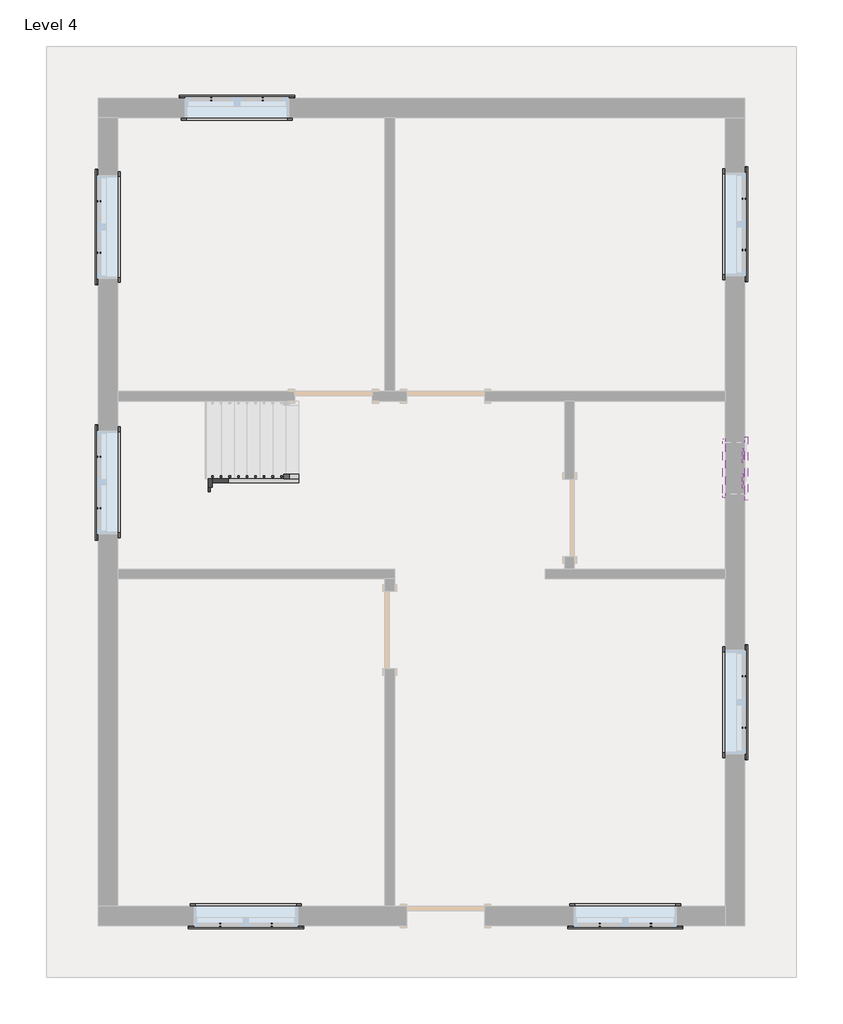
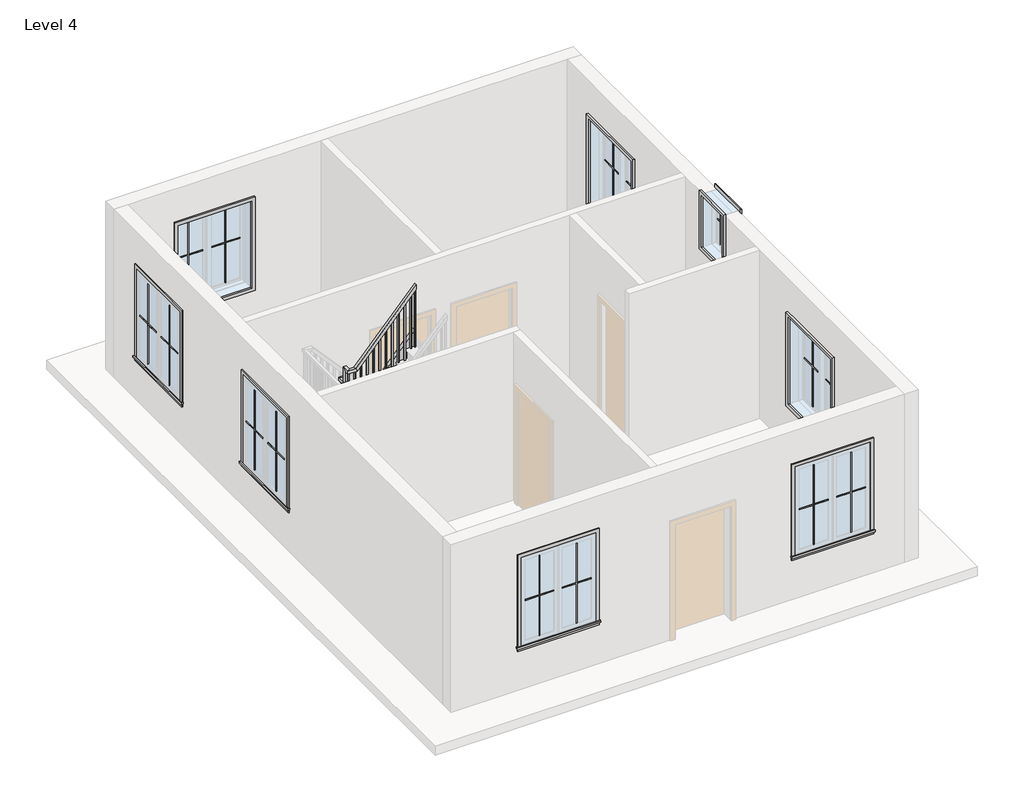
# One storey, part 2 of 2: 32 proxies, 3 members, 1 railing.
"""IFC4 building model written with IfcOpenShell, lengths in millimetres."""

from ifc_helpers import new_model, si_unit, frame, origin, place, context, project, spatial, polyline, outline, extrude, faceted_brep, transform, mapped, element, save
from components import muntin_pattern_2x2_muntin_pattern_2x2_6dad3731, muntin_pattern_2x2_muntin_pattern_2x2_a30a3345, muntin_pattern_2x2_muntin_pattern_2x2_53152e2c, muntin_pattern_2x2_muntin_pattern_2x2_e8f3e573, trim_window_exterior_flat_with_sill_92b9b949, trim_window_exterior_flat_with_sill_a665a915, trim_window_interior_flat_picture_frame_3bb882cf, trim_window_interior_flat_picture_frame_d485c387

model = new_model("IFC4")

# Units and contexts
model_context = context("Model", 3, world=origin())
ifc_project = project(units=[si_unit("LENGTHUNIT", "METRE", prefix="MILLI")], contexts=[model_context])

# Site, building, storey
site = spatial("IfcSite", under=ifc_project)
building = spatial("IfcBuilding", under=site)
storey = spatial("IfcBuildingStorey", under=building, Name="Level 4", Elevation=9144.0)

# Proxies
placement = place(None, origin())
muntin_pattern_2x2_muntin_pattern_2x2_shape = muntin_pattern_2x2_muntin_pattern_2x2_6dad3731(model_context)
element("IfcBuildingElementProxy", 1, Name="Muntin Pattern_2x2 : Muntin Pattern_2x2", ObjectType="Muntin Pattern_2x2 : Muntin Pattern_2x2", at=placement, inside=storey, context=model_context, shape_type="MappedRepresentation", body=[
    mapped(muntin_pattern_2x2_muntin_pattern_2x2_shape, transform((7785.1, 4733.925, 10128.25), x_axis=(-1.0, 0.0, 0.0), y_axis=(0.0, -1.0, 0.0), z_axis=(0.0, 0.0, 1.0))),
])
element("IfcBuildingElementProxy", 2, Name="Muntin Pattern_2x2 : Muntin Pattern_2x2", ObjectType="Muntin Pattern_2x2 : Muntin Pattern_2x2", at=placement, inside=storey, context=model_context, shape_type="MappedRepresentation", body=[
    mapped(muntin_pattern_2x2_muntin_pattern_2x2_shape, transform((3313.1125, 4733.925, 10128.25), x_axis=(-1.0, 0.0, 0.0), y_axis=(0.0, -1.0, 0.0), z_axis=(0.0, 0.0, 1.0))),
])
element("IfcBuildingElementProxy", 3, Name="Muntin Pattern_2x2 : Muntin Pattern_2x2", ObjectType="Muntin Pattern_2x2 : Muntin Pattern_2x2", at=placement, inside=storey, context=model_context, shape_type="MappedRepresentation", body=[
    mapped(muntin_pattern_2x2_muntin_pattern_2x2_shape, transform((8880.475, 13295.3125, 10128.25), x_axis=(0.0, -1.0, 0.0), y_axis=(1.0, 0.0, 0.0), z_axis=(0.0, 0.0, 1.0))),
])
element("IfcBuildingElementProxy", 4, Name="Muntin Pattern_2x2 : Muntin Pattern_2x2", ObjectType="Muntin Pattern_2x2 : Muntin Pattern_2x2", at=placement, inside=storey, context=model_context, shape_type="MappedRepresentation", body=[
    mapped(muntin_pattern_2x2_muntin_pattern_2x2_shape, transform((8880.475, 7662.8625, 10128.25), x_axis=(0.0, -1.0, 0.0), y_axis=(1.0, 0.0, 0.0), z_axis=(0.0, 0.0, 1.0))),
])
element("IfcBuildingElementProxy", 5, Name="Muntin Pattern_2x2 : Muntin Pattern_2x2", ObjectType="Muntin Pattern_2x2 : Muntin Pattern_2x2", at=placement, inside=storey, context=model_context, shape_type="MappedRepresentation", body=[
    mapped(muntin_pattern_2x2_muntin_pattern_2x2_shape, transform((1279.525, 12657.1375, 10128.25), x_axis=(0.0, 1.0, 0.0), y_axis=(-1.0, 0.0, 0.0), z_axis=(0.0, 0.0, 1.0))),
])
element("IfcBuildingElementProxy", 6, Name="Muntin Pattern_2x2 : Muntin Pattern_2x2", ObjectType="Muntin Pattern_2x2 : Muntin Pattern_2x2", at=placement, inside=storey, context=model_context, shape_type="MappedRepresentation", body=[
    mapped(muntin_pattern_2x2_muntin_pattern_2x2_shape, transform((1279.525, 9647.2375, 10128.25), x_axis=(0.0, 1.0, 0.0), y_axis=(-1.0, 0.0, 0.0), z_axis=(0.0, 0.0, 1.0))),
])
element("IfcBuildingElementProxy", 7, Name="Muntin Pattern_2x2 : Muntin Pattern_2x2", ObjectType="Muntin Pattern_2x2 : Muntin Pattern_2x2", at=placement, inside=storey, context=model_context, shape_type="MappedRepresentation", body=[
    mapped(muntin_pattern_2x2_muntin_pattern_2x2_shape, transform((2601.9125, 14468.475, 10128.25), x_axis=(1.0, 0.0, 0.0), y_axis=(0.0, 1.0, 0.0), z_axis=(0.0, 0.0, 1.0))),
])
muntin_pattern_2x2_muntin_pattern_2x2_2_shape = muntin_pattern_2x2_muntin_pattern_2x2_a30a3345(model_context)
element("IfcBuildingElementProxy", 8, Name="Muntin Pattern_2x2 : Muntin Pattern_2x2", ObjectType="Muntin Pattern_2x2 : Muntin Pattern_2x2", at=placement, inside=storey, context=model_context, shape_type="MappedRepresentation", body=[
    mapped(muntin_pattern_2x2_muntin_pattern_2x2_2_shape, transform((7178.675, 4733.925, 10128.25), x_axis=(1.0, 0.0, 0.0), y_axis=(0.0, 1.0, 0.0), z_axis=(0.0, 0.0, 1.0))),
])
element("IfcBuildingElementProxy", 9, Name="Muntin Pattern_2x2 : Muntin Pattern_2x2", ObjectType="Muntin Pattern_2x2 : Muntin Pattern_2x2", at=placement, inside=storey, context=model_context, shape_type="MappedRepresentation", body=[
    mapped(muntin_pattern_2x2_muntin_pattern_2x2_2_shape, transform((2706.6875, 4733.925, 10128.25), x_axis=(1.0, 0.0, 0.0), y_axis=(0.0, 1.0, 0.0), z_axis=(0.0, 0.0, 1.0))),
])
element("IfcBuildingElementProxy", 10, Name="Muntin Pattern_2x2 : Muntin Pattern_2x2", ObjectType="Muntin Pattern_2x2 : Muntin Pattern_2x2", at=placement, inside=storey, context=model_context, shape_type="MappedRepresentation", body=[
    mapped(muntin_pattern_2x2_muntin_pattern_2x2_2_shape, transform((8880.475, 12688.8875, 10128.25), x_axis=(0.0, 1.0, 0.0), y_axis=(-1.0, 0.0, 0.0), z_axis=(0.0, 0.0, 1.0))),
])
element("IfcBuildingElementProxy", 11, Name="Muntin Pattern_2x2 : Muntin Pattern_2x2", ObjectType="Muntin Pattern_2x2 : Muntin Pattern_2x2", at=placement, inside=storey, context=model_context, shape_type="MappedRepresentation", body=[
    mapped(muntin_pattern_2x2_muntin_pattern_2x2_2_shape, transform((8880.475, 7056.4375, 10128.25), x_axis=(0.0, 1.0, 0.0), y_axis=(-1.0, 0.0, 0.0), z_axis=(0.0, 0.0, 1.0))),
])
element("IfcBuildingElementProxy", 12, Name="Muntin Pattern_2x2 : Muntin Pattern_2x2", ObjectType="Muntin Pattern_2x2 : Muntin Pattern_2x2", at=placement, inside=storey, context=model_context, shape_type="MappedRepresentation", body=[
    mapped(muntin_pattern_2x2_muntin_pattern_2x2_2_shape, transform((1279.525, 13263.5625, 10128.25), x_axis=(0.0, -1.0, 0.0), y_axis=(1.0, 0.0, 0.0), z_axis=(0.0, 0.0, 1.0))),
])
element("IfcBuildingElementProxy", 13, Name="Muntin Pattern_2x2 : Muntin Pattern_2x2", ObjectType="Muntin Pattern_2x2 : Muntin Pattern_2x2", at=placement, inside=storey, context=model_context, shape_type="MappedRepresentation", body=[
    mapped(muntin_pattern_2x2_muntin_pattern_2x2_2_shape, transform((1279.525, 10253.6625, 10128.25), x_axis=(0.0, -1.0, 0.0), y_axis=(1.0, 0.0, 0.0), z_axis=(0.0, 0.0, 1.0))),
])
element("IfcBuildingElementProxy", 14, Name="Muntin Pattern_2x2 : Muntin Pattern_2x2", ObjectType="Muntin Pattern_2x2 : Muntin Pattern_2x2", at=placement, inside=storey, context=model_context, shape_type="MappedRepresentation", body=[
    mapped(muntin_pattern_2x2_muntin_pattern_2x2_2_shape, transform((3208.3375, 14468.475, 10128.25), x_axis=(-1.0, 0.0, 0.0), y_axis=(0.0, -1.0, 0.0), z_axis=(0.0, 0.0, 1.0))),
])
muntin_pattern_2x2_muntin_pattern_2x2_3_shape = muntin_pattern_2x2_muntin_pattern_2x2_53152e2c(model_context)
element("IfcBuildingElementProxy", 15, Name="Muntin Pattern_2x2 : Muntin Pattern_2x2", ObjectType="Muntin Pattern_2x2 : Muntin Pattern_2x2", at=placement, inside=storey, context=model_context, shape_type="MappedRepresentation", body=[
    mapped(muntin_pattern_2x2_muntin_pattern_2x2_3_shape, transform((8880.475, 10266.3625, 11347.45), x_axis=(0.0, -1.0, 0.0), y_axis=(1.0, 0.0, 0.0), z_axis=(0.0, 0.0, 1.0))),
])
muntin_pattern_2x2_muntin_pattern_2x2_4_shape = muntin_pattern_2x2_muntin_pattern_2x2_e8f3e573(model_context)
element("IfcBuildingElementProxy", 16, Name="Muntin Pattern_2x2 : Muntin Pattern_2x2", ObjectType="Muntin Pattern_2x2 : Muntin Pattern_2x2", at=placement, inside=storey, context=model_context, shape_type="MappedRepresentation", body=[
    mapped(muntin_pattern_2x2_muntin_pattern_2x2_4_shape, transform((8880.475, 9964.7375, 11347.45), x_axis=(0.0, 1.0, 0.0), y_axis=(-1.0, 0.0, 0.0), z_axis=(0.0, 0.0, 1.0))),
])
trim_window_exterior_flat_with_sill_shape = trim_window_exterior_flat_with_sill_92b9b949(model_context)
element("IfcBuildingElementProxy", 17, Name="Trim-Window-Exterior-Flat : with Sill", ObjectType="Trim-Window-Exterior-Flat : with Sill", at=placement, inside=storey, context=model_context, shape_type="MappedRepresentation", body=[
    mapped(trim_window_exterior_flat_with_sill_shape, transform((7481.8875, 4724.4, 11582.4), x_axis=(1.0, 0.0, 0.0), y_axis=(0.0, 0.0, 1.0), z_axis=(0.0, -1.0, 0.0))),
])
element("IfcBuildingElementProxy", 18, Name="Trim-Window-Exterior-Flat : with Sill", ObjectType="Trim-Window-Exterior-Flat : with Sill", at=placement, inside=storey, context=model_context, shape_type="MappedRepresentation", body=[
    mapped(trim_window_exterior_flat_with_sill_shape, transform((3009.9, 4724.4, 11582.4), x_axis=(1.0, 0.0, 0.0), y_axis=(0.0, 0.0, 1.0), z_axis=(0.0, -1.0, 0.0))),
])
element("IfcBuildingElementProxy", 19, Name="Trim-Window-Exterior-Flat : with Sill", ObjectType="Trim-Window-Exterior-Flat : with Sill", at=placement, inside=storey, context=model_context, shape_type="MappedRepresentation", body=[
    mapped(trim_window_exterior_flat_with_sill_shape, transform((8890.0, 12992.1, 11582.4), x_axis=(0.0, 1.0, 0.0), y_axis=(0.0, 0.0, 1.0), z_axis=(1.0, 0.0, 0.0))),
])
element("IfcBuildingElementProxy", 20, Name="Trim-Window-Exterior-Flat : with Sill", ObjectType="Trim-Window-Exterior-Flat : with Sill", at=placement, inside=storey, context=model_context, shape_type="MappedRepresentation", body=[
    mapped(trim_window_exterior_flat_with_sill_shape, transform((8890.0, 7359.65, 11582.4), x_axis=(0.0, 1.0, 0.0), y_axis=(0.0, 0.0, 1.0), z_axis=(1.0, 0.0, 0.0))),
])
element("IfcBuildingElementProxy", 21, Name="Trim-Window-Exterior-Flat : with Sill", ObjectType="Trim-Window-Exterior-Flat : with Sill", at=placement, inside=storey, context=model_context, shape_type="MappedRepresentation", body=[
    mapped(trim_window_exterior_flat_with_sill_shape, transform((1270.0, 12960.35, 11582.4), x_axis=(0.0, -1.0, 0.0), y_axis=(0.0, 0.0, 1.0), z_axis=(-1.0, 0.0, 0.0))),
])
element("IfcBuildingElementProxy", 22, Name="Trim-Window-Exterior-Flat : with Sill", ObjectType="Trim-Window-Exterior-Flat : with Sill", at=placement, inside=storey, context=model_context, shape_type="MappedRepresentation", body=[
    mapped(trim_window_exterior_flat_with_sill_shape, transform((1270.0, 9950.45, 11582.4), x_axis=(0.0, -1.0, 0.0), y_axis=(0.0, 0.0, 1.0), z_axis=(-1.0, 0.0, 0.0))),
])
element("IfcBuildingElementProxy", 23, Name="Trim-Window-Exterior-Flat : with Sill", ObjectType="Trim-Window-Exterior-Flat : with Sill", at=placement, inside=storey, context=model_context, shape_type="MappedRepresentation", body=[
    mapped(trim_window_exterior_flat_with_sill_shape, transform((2905.125, 14478.0, 11582.4), x_axis=(-1.0, 0.0, 0.0), y_axis=(0.0, 0.0, 1.0), z_axis=(0.0, 1.0, 0.0))),
])
trim_window_exterior_flat_with_sill_2_shape = trim_window_exterior_flat_with_sill_a665a915(model_context)
element("IfcBuildingElementProxy", 24, Name="Trim-Window-Exterior-Flat : with Sill", ObjectType="Trim-Window-Exterior-Flat : with Sill", at=placement, inside=storey, context=model_context, shape_type="MappedRepresentation", body=[
    mapped(trim_window_exterior_flat_with_sill_2_shape, transform((8890.0, 10115.55, 12192.0), x_axis=(0.0, 1.0, 0.0), y_axis=(0.0, 0.0, 1.0), z_axis=(1.0, 0.0, 0.0))),
])
trim_window_interior_flat_picture_frame_shape = trim_window_interior_flat_picture_frame_3bb882cf(model_context)
element("IfcBuildingElementProxy", 25, Name="Trim-Window-Interior-Flat : Picture Frame", ObjectType="Trim-Window-Interior-Flat : Picture Frame", at=placement, inside=storey, context=model_context, shape_type="MappedRepresentation", body=[
    mapped(trim_window_interior_flat_picture_frame_shape, transform((7481.8875, 4953.0, 11582.4), x_axis=(-1.0, 0.0, 0.0), y_axis=(0.0, 0.0, 1.0), z_axis=(0.0, 1.0, 0.0))),
])
element("IfcBuildingElementProxy", 26, Name="Trim-Window-Interior-Flat : Picture Frame", ObjectType="Trim-Window-Interior-Flat : Picture Frame", at=placement, inside=storey, context=model_context, shape_type="MappedRepresentation", body=[
    mapped(trim_window_interior_flat_picture_frame_shape, transform((3009.9, 4953.0, 11582.4), x_axis=(-1.0, 0.0, 0.0), y_axis=(0.0, 0.0, 1.0), z_axis=(0.0, 1.0, 0.0))),
])
element("IfcBuildingElementProxy", 27, Name="Trim-Window-Interior-Flat : Picture Frame", ObjectType="Trim-Window-Interior-Flat : Picture Frame", at=placement, inside=storey, context=model_context, shape_type="MappedRepresentation", body=[
    mapped(trim_window_interior_flat_picture_frame_shape, transform((8661.4, 12992.1, 11582.4), x_axis=(0.0, -1.0, 0.0), y_axis=(0.0, 0.0, 1.0), z_axis=(-1.0, 0.0, 0.0))),
])
element("IfcBuildingElementProxy", 28, Name="Trim-Window-Interior-Flat : Picture Frame", ObjectType="Trim-Window-Interior-Flat : Picture Frame", at=placement, inside=storey, context=model_context, shape_type="MappedRepresentation", body=[
    mapped(trim_window_interior_flat_picture_frame_shape, transform((8661.4, 7359.65, 11582.4), x_axis=(0.0, -1.0, 0.0), y_axis=(0.0, 0.0, 1.0), z_axis=(-1.0, 0.0, 0.0))),
])
element("IfcBuildingElementProxy", 29, Name="Trim-Window-Interior-Flat : Picture Frame", ObjectType="Trim-Window-Interior-Flat : Picture Frame", at=placement, inside=storey, context=model_context, shape_type="MappedRepresentation", body=[
    mapped(trim_window_interior_flat_picture_frame_shape, transform((1498.6, 12960.35, 11582.4), x_axis=(0.0, 1.0, 0.0), y_axis=(0.0, 0.0, 1.0), z_axis=(1.0, 0.0, 0.0))),
])
element("IfcBuildingElementProxy", 30, Name="Trim-Window-Interior-Flat : Picture Frame", ObjectType="Trim-Window-Interior-Flat : Picture Frame", at=placement, inside=storey, context=model_context, shape_type="MappedRepresentation", body=[
    mapped(trim_window_interior_flat_picture_frame_shape, transform((1498.6, 9950.45, 11582.4), x_axis=(0.0, 1.0, 0.0), y_axis=(0.0, 0.0, 1.0), z_axis=(1.0, 0.0, 0.0))),
])
element("IfcBuildingElementProxy", 31, Name="Trim-Window-Interior-Flat : Picture Frame", ObjectType="Trim-Window-Interior-Flat : Picture Frame", at=placement, inside=storey, context=model_context, shape_type="MappedRepresentation", body=[
    mapped(trim_window_interior_flat_picture_frame_shape, transform((2905.125, 14249.4, 11582.4), x_axis=(1.0, 0.0, 0.0), y_axis=(0.0, 0.0, 1.0), z_axis=(0.0, -1.0, 0.0))),
])
trim_window_interior_flat_picture_frame_2_shape = trim_window_interior_flat_picture_frame_d485c387(model_context)
element("IfcBuildingElementProxy", 32, Name="Trim-Window-Interior-Flat : Picture Frame", ObjectType="Trim-Window-Interior-Flat : Picture Frame", at=placement, inside=storey, context=model_context, shape_type="MappedRepresentation", body=[
    mapped(trim_window_interior_flat_picture_frame_2_shape, transform((8661.4, 10115.55, 12192.0), x_axis=(0.0, -1.0, 0.0), y_axis=(0.0, 0.0, 1.0), z_axis=(-1.0, 0.0, 0.0))),
])

# Members
element("IfcMember", 33, ObjectType="Stringer - 2\" Width", at=placement, inside=storey, context=model_context, shape_type="SweptSolid", body=[
    extrude(outline(polyline([(9144.0, 3632.2), (9418.6288314, 3632.2), (10547.5177203, 2616.2), (10091.8883192, 2616.2), (9144.0, 3469.2994873), (9144.0, 3632.2)])), frame((0.0, 9944.1, 0.0), z_axis=(0.0, 1.0, 0.0), x_axis=(0.0, 0.0, 1.0)), (0.0, 0.0, 1.0), 50.8),
])
element("IfcMember", 34, ObjectType="Stringer - 2\" Width", at=placement, inside=storey, context=model_context, shape_type="SweptSolid", body=[
    extrude(outline(polyline([(2565.4, 9994.9), (2616.2, 9994.9), (2616.2, 9893.3), (2565.4, 9893.3), (2565.4, 9994.9)])), frame((0.0, 0.0, 10270.0666667), z_axis=(0.0, 0.0, 1.0), x_axis=(1.0, 0.0, 0.0)), (0.0, 0.0, 1.0), 304.8),
])
element("IfcMember", 35, ObjectType="Stringer - 2\" Width", at=placement, inside=storey, context=model_context, shape_type="SweptSolid", body=[
    extrude(outline(polyline([(10773.2954981, 2565.4), (10317.666097, 2565.4), (11502.9994303, 3632.2), (11958.6288314, 3632.2), (10773.2954981, 2565.4)])), frame((0.0, 9842.5, 0.0), z_axis=(0.0, 1.0, 0.0), x_axis=(0.0, 0.0, 1.0)), (0.0, 0.0, 1.0), 50.8),
])

# Railing
element("IfcRailing", 36, ObjectType="Handrail - Rectangular", at=placement, inside=storey, context=model_context, shape_type="SolidModel", body=[
    faceted_brep([(3632.2, 9994.9, 10227.7333333), (3632.2, 9994.9, 10151.7950998), (3632.2, 10045.7, 10151.7950998), (3632.2, 10045.7, 10227.7333333), (2641.6, 9994.9, 11328.4), (2590.8, 9994.9, 11308.9062109), (2590.8, 10045.7, 11308.9062109), (2641.6, 10045.7, 11328.4), (2641.6, 9994.9, 11413.0666667), (2590.8, 9994.9, 11362.2666667), (2590.8, 10045.7, 11362.2666667), (2641.6, 10045.7, 11413.0666667), (2565.4, 9994.9, 11413.0666667), (2565.4, 9994.9, 11362.2666667), (2514.6, 10045.7, 11362.2666667), (2514.6, 10045.7, 11413.0666667), (2565.4, 9918.7, 11413.0666667), (2565.4, 9867.9, 11362.2666667), (2514.6, 9867.9, 11362.2666667), (2514.6, 9918.7, 11413.0666667), (2565.4, 9918.7, 11667.0666667), (2565.4, 9867.9, 11616.2666667), (2514.6, 9867.9, 11616.2666667), (2514.6, 9918.7, 11667.0666667), (2565.4, 9842.5, 11667.0666667), (2565.4, 9842.5, 11616.2666667), (2514.6, 9791.7, 11616.2666667), (2514.6, 9791.7, 11667.0666667), (2641.6, 9842.5, 11667.0666667), (2664.2244102, 9842.5, 11616.2666667), (2664.2244102, 9791.7, 11616.2666667), (2641.6, 9791.7, 11667.0666667), (3632.2, 9842.5, 12767.7333333), (3632.2, 9791.7, 12767.7333333), (3632.2, 9791.7, 12691.7950998), (3632.2, 9842.5, 12691.7950998)], [[[0, 1, 2, 3]], [[1, 0, 4, 5]], [[2, 1, 5, 6]], [[3, 2, 6, 7]], [[0, 3, 7, 4]], [[5, 4, 8, 9]], [[6, 5, 9, 10]], [[7, 6, 10, 11]], [[4, 7, 11, 8]], [[9, 8, 12, 13]], [[10, 9, 13, 14]], [[11, 10, 14, 15]], [[8, 11, 15, 12]], [[13, 12, 16, 17]], [[14, 13, 17, 18]], [[15, 14, 18, 19]], [[12, 15, 19, 16]], [[17, 16, 20, 21]], [[18, 17, 21, 22]], [[19, 18, 22, 23]], [[16, 19, 23, 20]], [[21, 20, 24, 25]], [[22, 21, 25, 26]], [[23, 22, 26, 27]], [[20, 23, 27, 24]], [[25, 24, 28, 29]], [[26, 25, 29, 30]], [[27, 26, 30, 31]], [[24, 27, 31, 28]], [[32, 33, 34, 35]], [[29, 28, 32, 35]], [[30, 29, 35, 34]], [[31, 30, 34, 33]], [[28, 31, 33, 32]]]),
    extrude(outline(polyline([(12596.5450998, 3546.475), (11684.0, 3546.475), (11684.0, 3565.525), (12617.7117665, 3565.525), (12596.5450998, 3546.475)])), frame((0.0, 9807.575, 0.0), z_axis=(0.0, 1.0, 0.0), x_axis=(0.0, 0.0, 1.0)), (0.0, 0.0, 1.0), 19.05),
    extrude(outline(polyline([(12483.6562109, 3444.875), (11514.6666667, 3444.875), (11514.6666667, 3463.925), (12504.8228776, 3463.925), (12483.6562109, 3444.875)])), frame((0.0, 9807.575, 0.0), z_axis=(0.0, 1.0, 0.0), x_axis=(0.0, 0.0, 1.0)), (0.0, 0.0, 1.0), 19.05),
    extrude(outline(polyline([(12370.767322, 3343.275), (11514.6666667, 3343.275), (11514.6666667, 3362.325), (12391.9339887, 3362.325), (12370.767322, 3343.275)])), frame((0.0, 9807.575, 0.0), z_axis=(0.0, 1.0, 0.0), x_axis=(0.0, 0.0, 1.0)), (0.0, 0.0, 1.0), 19.05),
    extrude(outline(polyline([(12257.8784332, 3241.675), (11345.3333333, 3241.675), (11345.3333333, 3260.725), (12279.0450998, 3260.725), (12257.8784332, 3241.675)])), frame((0.0, 9807.575, 0.0), z_axis=(0.0, 1.0, 0.0), x_axis=(0.0, 0.0, 1.0)), (0.0, 0.0, 1.0), 19.05),
    extrude(outline(polyline([(12144.9895443, 3140.075), (11176.0, 3140.075), (11176.0, 3159.125), (12166.1562109, 3159.125), (12144.9895443, 3140.075)])), frame((0.0, 9807.575, 0.0), z_axis=(0.0, 1.0, 0.0), x_axis=(0.0, 0.0, 1.0)), (0.0, 0.0, 1.0), 19.05),
    extrude(outline(polyline([(12032.1006554, 3038.475), (11176.0, 3038.475), (11176.0, 3057.525), (12053.267322, 3057.525), (12032.1006554, 3038.475)])), frame((0.0, 9807.575, 0.0), z_axis=(0.0, 1.0, 0.0), x_axis=(0.0, 0.0, 1.0)), (0.0, 0.0, 1.0), 19.05),
    extrude(outline(polyline([(11919.2117665, 2936.875), (11006.6666667, 2936.875), (11006.6666667, 2955.925), (11940.3784332, 2955.925), (11919.2117665, 2936.875)])), frame((0.0, 9807.575, 0.0), z_axis=(0.0, 1.0, 0.0), x_axis=(0.0, 0.0, 1.0)), (0.0, 0.0, 1.0), 19.05),
    extrude(outline(polyline([(11806.3228776, 2835.275), (10837.3333333, 2835.275), (10837.3333333, 2854.325), (11827.4895443, 2854.325), (11806.3228776, 2835.275)])), frame((0.0, 9807.575, 0.0), z_axis=(0.0, 1.0, 0.0), x_axis=(0.0, 0.0, 1.0)), (0.0, 0.0, 1.0), 19.05),
    extrude(outline(polyline([(11693.4339887, 2733.675), (10837.3333333, 2733.675), (10837.3333333, 2752.725), (11714.6006554, 2752.725), (11693.4339887, 2733.675)])), frame((0.0, 9807.575, 0.0), z_axis=(0.0, 1.0, 0.0), x_axis=(0.0, 0.0, 1.0)), (0.0, 0.0, 1.0), 19.05),
    extrude(outline(polyline([(11580.5450998, 2632.075), (10668.0, 2632.075), (10668.0, 2651.125), (11601.7117665, 2651.125), (11580.5450998, 2632.075)])), frame((0.0, 9807.575, 0.0), z_axis=(0.0, 1.0, 0.0), x_axis=(0.0, 0.0, 1.0)), (0.0, 0.0, 1.0), 19.05),
    extrude(outline(polyline([(2549.525, 9928.225), (2549.525, 9909.175), (2530.475, 9909.175), (2530.475, 9928.225), (2549.525, 9928.225)])), frame((0.0, 0.0, 10498.6666667), z_axis=(0.0, 0.0, 1.0), x_axis=(1.0, 0.0, 0.0)), (0.0, 0.0, 1.0), 863.6),
    extrude(outline(polyline([(2625.725, 10010.775), (2606.675, 10010.775), (2606.675, 10029.825), (2625.725, 10029.825), (2625.725, 10010.775)])), frame((0.0, 0.0, 10329.3333333), z_axis=(0.0, 0.0, 1.0), x_axis=(1.0, 0.0, 0.0)), (0.0, 0.0, 1.0), 1032.9333333),
    extrude(outline(polyline([(11178.3784332, 2708.275), (10329.3333333, 2708.275), (10329.3333333, 2727.325), (11157.2117665, 2727.325), (11178.3784332, 2708.275)])), frame((0.0, 10010.775, 0.0), z_axis=(0.0, 1.0, 0.0), x_axis=(0.0, 0.0, 1.0)), (0.0, 0.0, 1.0), 19.05),
    extrude(outline(polyline([(11065.4895443, 2809.875), (10160.0, 2809.875), (10160.0, 2828.925), (11044.3228776, 2828.925), (11065.4895443, 2809.875)])), frame((0.0, 10010.775, 0.0), z_axis=(0.0, 1.0, 0.0), x_axis=(0.0, 0.0, 1.0)), (0.0, 0.0, 1.0), 19.05),
    extrude(outline(polyline([(10952.6006554, 2911.475), (9990.6666667, 2911.475), (9990.6666667, 2930.525), (10931.4339887, 2930.525), (10952.6006554, 2911.475)])), frame((0.0, 10010.775, 0.0), z_axis=(0.0, 1.0, 0.0), x_axis=(0.0, 0.0, 1.0)), (0.0, 0.0, 1.0), 19.05),
    extrude(outline(polyline([(10839.7117665, 3013.075), (9990.6666667, 3013.075), (9990.6666667, 3032.125), (10818.5450998, 3032.125), (10839.7117665, 3013.075)])), frame((0.0, 10010.775, 0.0), z_axis=(0.0, 1.0, 0.0), x_axis=(0.0, 0.0, 1.0)), (0.0, 0.0, 1.0), 19.05),
    extrude(outline(polyline([(10726.8228776, 3114.675), (9821.3333333, 3114.675), (9821.3333333, 3133.725), (10705.6562109, 3133.725), (10726.8228776, 3114.675)])), frame((0.0, 10010.775, 0.0), z_axis=(0.0, 1.0, 0.0), x_axis=(0.0, 0.0, 1.0)), (0.0, 0.0, 1.0), 19.05),
    extrude(outline(polyline([(10613.9339887, 3216.275), (9652.0, 3216.275), (9652.0, 3235.325), (10592.767322, 3235.325), (10613.9339887, 3216.275)])), frame((0.0, 10010.775, 0.0), z_axis=(0.0, 1.0, 0.0), x_axis=(0.0, 0.0, 1.0)), (0.0, 0.0, 1.0), 19.05),
    extrude(outline(polyline([(10501.0450998, 3317.875), (9652.0, 3317.875), (9652.0, 3336.925), (10479.8784332, 3336.925), (10501.0450998, 3317.875)])), frame((0.0, 10010.775, 0.0), z_axis=(0.0, 1.0, 0.0), x_axis=(0.0, 0.0, 1.0)), (0.0, 0.0, 1.0), 19.05),
    extrude(outline(polyline([(10388.1562109, 3419.475), (9482.6666667, 3419.475), (9482.6666667, 3438.525), (10366.9895443, 3438.525), (10388.1562109, 3419.475)])), frame((0.0, 10010.775, 0.0), z_axis=(0.0, 1.0, 0.0), x_axis=(0.0, 0.0, 1.0)), (0.0, 0.0, 1.0), 19.05),
    extrude(outline(polyline([(10275.267322, 3521.075), (9313.3333333, 3521.075), (9313.3333333, 3540.125), (10254.1006554, 3540.125), (10275.267322, 3521.075)])), frame((0.0, 10010.775, 0.0), z_axis=(0.0, 1.0, 0.0), x_axis=(0.0, 0.0, 1.0)), (0.0, 0.0, 1.0), 19.05),
    extrude(outline(polyline([(2549.525, 9826.625), (2549.525, 9807.575), (2530.475, 9807.575), (2530.475, 9826.625), (2549.525, 9826.625)])), frame((0.0, 0.0, 10498.6666667), z_axis=(0.0, 0.0, 1.0), x_axis=(1.0, 0.0, 0.0)), (0.0, 0.0, 1.0), 1117.6),
    extrude(outline(polyline([(2549.525, 10010.775), (2530.475, 10010.775), (2530.475, 10029.825), (2549.525, 10029.825), (2549.525, 10010.775)])), frame((0.0, 0.0, 10498.6666667), z_axis=(0.0, 0.0, 1.0), x_axis=(1.0, 0.0, 0.0)), (0.0, 0.0, 1.0), 863.6),
    extrude(outline(polyline([(12670.6284332, 3613.15), (11684.0, 3613.15), (11684.0, 3632.2), (12691.7950998, 3632.2), (12670.6284332, 3613.15)])), frame((0.0, 9807.575, 0.0), z_axis=(0.0, 1.0, 0.0), x_axis=(0.0, 0.0, 1.0)), (0.0, 0.0, 1.0), 19.05),
    extrude(outline(polyline([(10172.9617665, 3613.15), (9313.3333333, 3613.15), (9313.3333333, 3632.2), (10151.7950998, 3632.2), (10172.9617665, 3613.15)])), frame((0.0, 10010.775, 0.0), z_axis=(0.0, 1.0, 0.0), x_axis=(0.0, 0.0, 1.0)), (0.0, 0.0, 1.0), 19.05),
])

save(model, "model.ifc")

# Revit data of these elements
# Type "Muntin Pattern_2x2 : Muntin Pattern_2x2"
#   Width [instance default] = 4' - 0"
#   Thickness = 0' - 0 1/2"
#   Height [instance default] = 4' - 0"
#   Distance = 0' - 0 3/4"
#   Interior Material [instance default] = none
#   Exterior Material [instance default] = none
#   Default Elevation = 0
# Type "Trim-Window-Exterior-Flat : with Sill"
#   Trim Width = 0' - 2 1/4"
#   Trim Thickness_Picture Frame = 0' - 1 1/4"
#   Trim Thickness_with Sill = 0' - 0 3/4"
#   Sill Thickness = 0' - 1 1/4"
#   Opening Width [instance default] = 2' - 0"
#   Opening Height [instance default] = 3' - 0"
#   Default Elevation = 4' - 0"
#   Sill = yes
#   Picture Frame = no
#   Trim Material [instance default] = none
# Type "Trim-Window-Interior-Flat : Picture Frame"
#   Trim Thickness_Picture Frame = 0' - 1 1/4"
#   Trim Width = 0' - 2 1/4"
#   Trim Thickness_with Sill = 0' - 0 3/4"
#   Sill Thickness = 0' - 1 1/4"
#   Opening Width [instance default] = 2' - 0"
#   Opening Height [instance default] = 3' - 0"
#   Default Elevation = 4' - 0"
#   Sill = no
#   Picture Frame = yes
#   Trim Material [instance default] = none
# Type "Handrail - Rectangular"
#   Assembly Code = "C2010400"
#   built-in parameter 1008612 = 0.0416667 (stored number, unit not read)
#   built-in parameter 1008611 = 0.0416667 (stored number, unit not read)
#   built-in parameter 1008609 = 0.333333 (stored number, unit not read)
#   built-in parameter 1008604 = 0.166667 (stored number, unit not read)
#   built-in parameter 1008603 = 0.166667 (stored number, unit not read)
#   Railing Height = 3' - 0"
#   built-in parameter 1008630 = 2
#   built-in parameter 1008610 = 2
#   built-in parameter 1008618 = Baluster - Square : 3/4"
# Elements 1, 2, 3, 4, 5, 6, 7, 8, 9, 10, 11, 12, 13, 14 (IfcBuildingElementProxy, "Muntin Pattern_2x2 : Muntin Pattern_2x2")
#   Width = 1' - 6 5/8"
#   Height = 4' - 6 1/2"
#   Interior Material = Wood - Stained
#   Exterior Material = Clad - White
#   Phase Created = New Construction
#   Materials on its faces: "Clad - White", "Wood - Stained"
# Elements 15, 16 (IfcBuildingElementProxy, "Muntin Pattern_2x2 : Muntin Pattern_2x2")
#   Width = 0' - 6 5/8"
#   Height = 2' - 6 1/2"
#   Interior Material = Wood - Stained
#   Exterior Material = Clad - White
#   Phase Created = New Construction
#   Materials on its faces: "Clad - White", "Wood - Stained"
# Elements 17, 18, 19, 20, 21, 22, 23 (IfcBuildingElementProxy, "Trim-Window-Exterior-Flat : with Sill")
#   Opening Width = 4' - 0"
#   Opening Height = 5' - 0"
#   Trim Material = Clad - White
#   Phase Created = New Construction
#   Materials on its faces: "Clad - White"
# Element 24 (IfcBuildingElementProxy, "Trim-Window-Exterior-Flat : with Sill")
#   Opening Width = 2' - 0"
#   Opening Height = 3' - 0"
#   Trim Material = Clad - White
#   Phase Created = New Construction
#   Materials on its faces: "Clad - White"
# Elements 25, 26, 27, 28, 29, 30, 31 (IfcBuildingElementProxy, "Trim-Window-Interior-Flat : Picture Frame")
#   Opening Width = 4' - 0"
#   Opening Height = 5' - 0"
#   Trim Material = Wood - Stained
#   Phase Created = New Construction
#   Materials on its faces: "Wood - Stained"
# Element 32 (IfcBuildingElementProxy, "Trim-Window-Interior-Flat : Picture Frame")
#   Opening Width = 2' - 0"
#   Opening Height = 3' - 0"
#   Trim Material = Wood - Stained
#   Phase Created = New Construction
#   Materials on its faces: "Wood - Stained"
# Elements 33, 34, 35 (IfcMember, "Stringer - 2\" Width")
#   Phase Created = New Construction
# Element 36 (IfcRailing, "Handrail - Rectangular")
#   Phase Created = New Construction
# Materials
#   "Clad - White": class "Wood", colour RGB 242 242 238, transparency 0, Cost = 0
#   "Wood - Stained": class "Wood", colour RGB 224 178 126, transparency 0, Cost = 0
